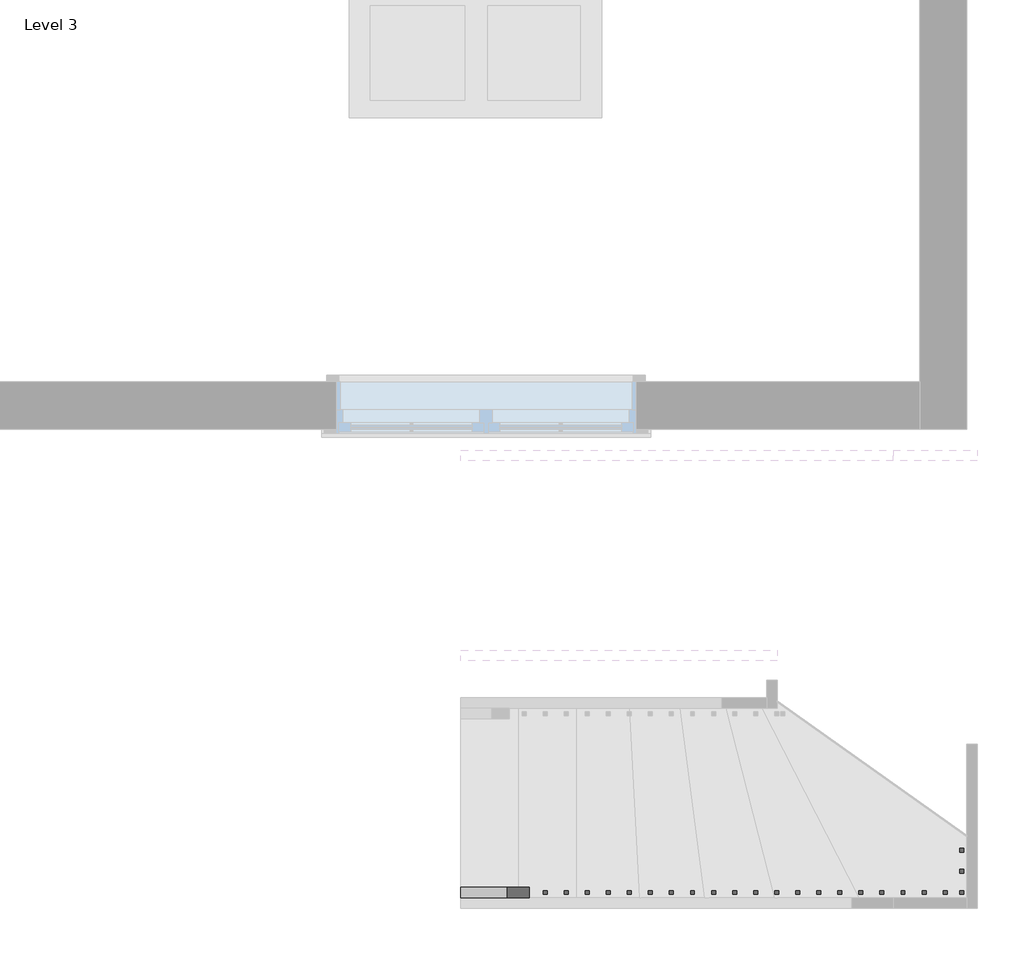
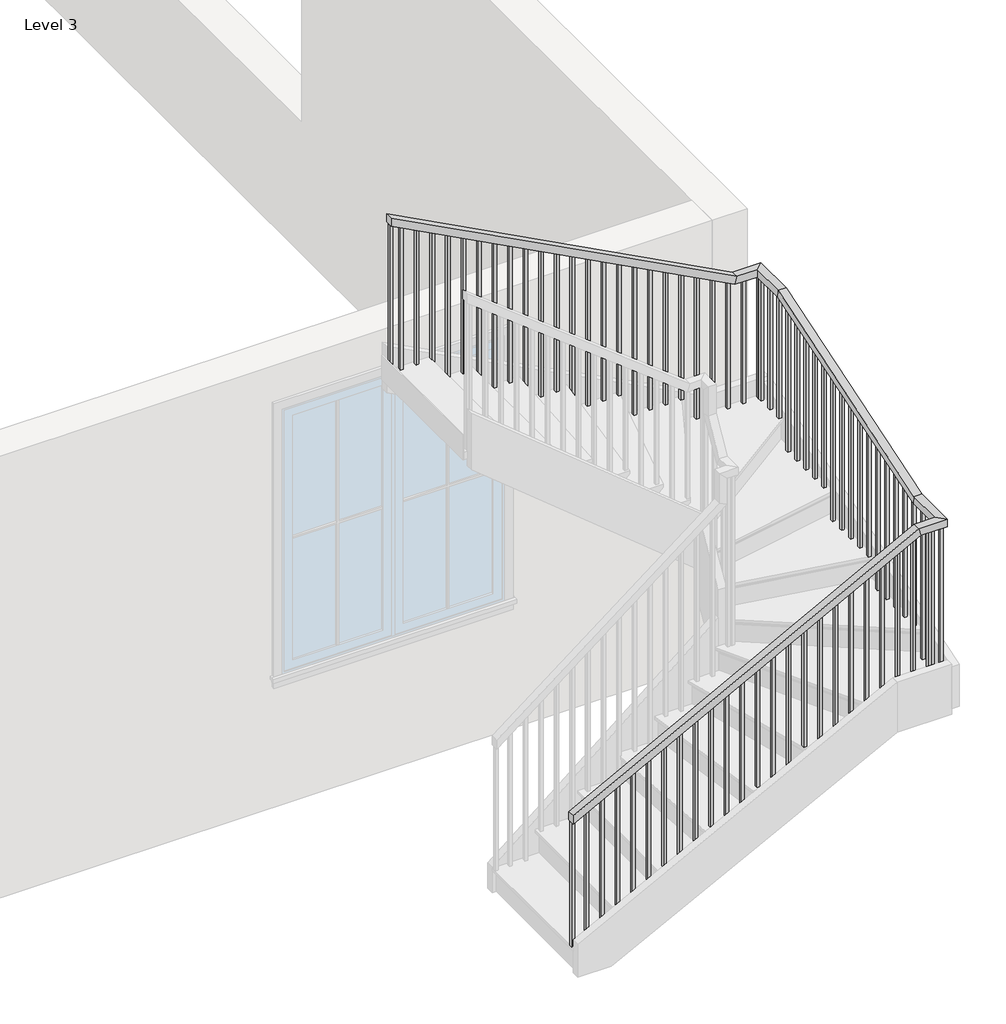
# One storey, part 2 of 3: 1 railing.
"""IFC4 building model written with IfcOpenShell, lengths in millimetres."""

from ifc_helpers import new_model, si_unit, frame, origin, place, context, project, spatial, polyline, outline, extrude, faceted_brep, element, save

model = new_model("IFC4")

# Units and contexts
model_context = context("Model", 3, world=origin())
ifc_project = project(units=[si_unit("LENGTHUNIT", "METRE", prefix="MILLI")], contexts=[model_context])

# Site, building, storey
site = spatial("IfcSite", under=ifc_project)
building = spatial("IfcBuilding", under=site)
storey = spatial("IfcBuildingStorey", under=building, Name="Level 3", Elevation=3200.4)

# Railing
placement = place(None, origin())
element("IfcRailing", 1, ObjectType="Handrail - Rectangular", at=placement, inside=storey, context=model_context, shape_type="SolidModel", body=[
    faceted_brep([(531.7538115, -7514.4090409, 4284.1333333), (531.7538115, -7514.4090409, 4226.6742652), (531.7538115, -7565.2090409, 4226.6742652), (531.7538115, -7565.2090409, 4284.1333333), (2789.4788736, -7514.4090409, 5477.4239201), (2802.0779381, -7514.4090409, 5426.6239201), (2802.0779381, -7565.2090409, 5426.6239201), (2789.4788736, -7565.2090409, 5477.4239201), (2923.0855034, -7269.9465826, 5426.6239201), (2923.0855034, -7277.8971587, 5477.4239201), (2923.0855034, -5744.320923, 5969.5094132), (2923.0855034, -5736.3703469, 5918.7094132), (2973.8855034, -7269.9465826, 5426.6239201), (2973.8855034, -5736.3703469, 5918.7094132), (2973.8855034, -7277.8971587, 5477.4239201), (2973.8855034, -5744.320923, 5969.5094132), (531.7538115, -5507.8090409, 7162.8), (531.7538115, -5457.0090409, 7162.8), (531.7538115, -5457.0090409, 7105.3409318), (531.7538115, -5507.8090409, 7105.3409318), (2776.879809, -5507.8090409, 5918.7094132), (2789.4788736, -5507.8090409, 5969.5094132), (2776.879809, -5457.0090409, 5918.7094132), (2789.4788736, -5457.0090409, 5969.5094132), (2923.0855034, -7514.4090409, 5477.4239201), (2923.0855034, -7514.4090409, 5426.6239201), (2973.8855034, -7565.2090409, 5426.6239201), (2973.8855034, -7565.2090409, 5477.4239201), (2923.0855034, -5507.8090409, 5969.5094132), (2923.0855034, -5507.8090409, 5918.7094132), (2973.8855034, -5457.0090409, 5918.7094132), (2973.8855034, -5457.0090409, 5969.5094132)], [[[0, 1, 2, 3]], [[1, 0, 4, 5]], [[2, 1, 5, 6]], [[3, 2, 6, 7]], [[0, 3, 7, 4]], [[8, 9, 10, 11]], [[12, 8, 11, 13]], [[14, 12, 13, 15]], [[9, 14, 15, 10]], [[16, 17, 18, 19]], [[20, 21, 16, 19]], [[22, 20, 19, 18]], [[23, 22, 18, 17]], [[21, 23, 17, 16]], [[5, 4, 24, 25]], [[6, 5, 25, 26]], [[7, 6, 26, 27]], [[4, 7, 27, 24]], [[25, 24, 9, 8]], [[26, 25, 8, 12]], [[27, 26, 12, 14]], [[24, 27, 14, 9]], [[11, 10, 28, 29]], [[13, 11, 29, 30]], [[15, 13, 30, 31]], [[10, 15, 31, 28]], [[29, 28, 21, 20]], [[30, 29, 20, 22]], [[31, 30, 22, 23]], [[28, 31, 23, 21]]]),
    extrude(outline(polyline([(7058.0597858, 621.2105034), (7068.1284102, 602.1605034), (6079.0666667, 602.1605034), (6079.0666667, 621.2105034), (7058.0597858, 621.2105034)])), frame((0.0, -5491.9340409, 0.0), z_axis=(0.0, 1.0, 0.0), x_axis=(0.0, 0.0, 1.0)), (0.0, 0.0, 1.0), 19.05),
    extrude(outline(polyline([(7004.3604556, 722.8105034), (7014.42908, 703.7605034), (6079.0666667, 703.7605034), (6079.0666667, 722.8105034), (7004.3604556, 722.8105034)])), frame((0.0, -5491.9340409, 0.0), z_axis=(0.0, 1.0, 0.0), x_axis=(0.0, 0.0, 1.0)), (0.0, 0.0, 1.0), 19.05),
    extrude(outline(polyline([(6950.6611254, 824.4105034), (6960.7297498, 805.3605034), (5909.7333333, 805.3605034), (5909.7333333, 824.4105034), (6950.6611254, 824.4105034)])), frame((0.0, -5491.9340409, 0.0), z_axis=(0.0, 1.0, 0.0), x_axis=(0.0, 0.0, 1.0)), (0.0, 0.0, 1.0), 19.05),
    extrude(outline(polyline([(6896.9617952, 926.0105034), (6907.0304196, 906.9605034), (5909.7333333, 906.9605034), (5909.7333333, 926.0105034), (6896.9617952, 926.0105034)])), frame((0.0, -5491.9340409, 0.0), z_axis=(0.0, 1.0, 0.0), x_axis=(0.0, 0.0, 1.0)), (0.0, 0.0, 1.0), 19.05),
    extrude(outline(polyline([(6843.262465, 1027.6105034), (6853.3310894, 1008.5605034), (5909.7333333, 1008.5605034), (5909.7333333, 1027.6105034), (6843.262465, 1027.6105034)])), frame((0.0, -5491.9340409, 0.0), z_axis=(0.0, 1.0, 0.0), x_axis=(0.0, 0.0, 1.0)), (0.0, 0.0, 1.0), 19.05),
    extrude(outline(polyline([(6789.5631348, 1129.2105034), (6799.6317592, 1110.1605034), (5740.4, 1110.1605034), (5740.4, 1129.2105034), (6789.5631348, 1129.2105034)])), frame((0.0, -5491.9340409, 0.0), z_axis=(0.0, 1.0, 0.0), x_axis=(0.0, 0.0, 1.0)), (0.0, 0.0, 1.0), 19.05),
    extrude(outline(polyline([(6735.8638046, 1230.8105034), (6745.932429, 1211.7605034), (5740.4, 1211.7605034), (5740.4, 1230.8105034), (6735.8638046, 1230.8105034)])), frame((0.0, -5491.9340409, 0.0), z_axis=(0.0, 1.0, 0.0), x_axis=(0.0, 0.0, 1.0)), (0.0, 0.0, 1.0), 19.05),
    extrude(outline(polyline([(6682.1644744, 1332.4105034), (6692.2330988, 1313.3605034), (5740.4, 1313.3605034), (5740.4, 1332.4105034), (6682.1644744, 1332.4105034)])), frame((0.0, -5491.9340409, 0.0), z_axis=(0.0, 1.0, 0.0), x_axis=(0.0, 0.0, 1.0)), (0.0, 0.0, 1.0), 19.05),
    extrude(outline(polyline([(6628.4651442, 1434.0105034), (6638.5337686, 1414.9605034), (5571.0666667, 1414.9605034), (5571.0666667, 1434.0105034), (6628.4651442, 1434.0105034)])), frame((0.0, -5491.9340409, 0.0), z_axis=(0.0, 1.0, 0.0), x_axis=(0.0, 0.0, 1.0)), (0.0, 0.0, 1.0), 19.05),
    extrude(outline(polyline([(6574.765814, 1535.6105034), (6584.8344384, 1516.5605034), (5571.0666667, 1516.5605034), (5571.0666667, 1535.6105034), (6574.765814, 1535.6105034)])), frame((0.0, -5491.9340409, 0.0), z_axis=(0.0, 1.0, 0.0), x_axis=(0.0, 0.0, 1.0)), (0.0, 0.0, 1.0), 19.05),
    extrude(outline(polyline([(6521.0664838, 1637.2105034), (6531.1351082, 1618.1605034), (5571.0666667, 1618.1605034), (5571.0666667, 1637.2105034), (6521.0664838, 1637.2105034)])), frame((0.0, -5491.9340409, 0.0), z_axis=(0.0, 1.0, 0.0), x_axis=(0.0, 0.0, 1.0)), (0.0, 0.0, 1.0), 19.05),
    extrude(outline(polyline([(6467.3671536, 1738.8105034), (6477.435778, 1719.7605034), (5401.7333333, 1719.7605034), (5401.7333333, 1738.8105034), (6467.3671536, 1738.8105034)])), frame((0.0, -5491.9340409, 0.0), z_axis=(0.0, 1.0, 0.0), x_axis=(0.0, 0.0, 1.0)), (0.0, 0.0, 1.0), 19.05),
    extrude(outline(polyline([(6413.6678234, 1840.4105034), (6423.7364478, 1821.3605034), (5401.7333333, 1821.3605034), (5401.7333333, 1840.4105034), (6413.6678234, 1840.4105034)])), frame((0.0, -5491.9340409, 0.0), z_axis=(0.0, 1.0, 0.0), x_axis=(0.0, 0.0, 1.0)), (0.0, 0.0, 1.0), 19.05),
    extrude(outline(polyline([(6359.9684932, 1942.0105034), (6370.0371176, 1922.9605034), (5401.7333333, 1922.9605034), (5401.7333333, 1942.0105034), (6359.9684932, 1942.0105034)])), frame((0.0, -5491.9340409, 0.0), z_axis=(0.0, 1.0, 0.0), x_axis=(0.0, 0.0, 1.0)), (0.0, 0.0, 1.0), 19.05),
    extrude(outline(polyline([(6306.269163, 2043.6105034), (6316.3377874, 2024.5605034), (5401.7333333, 2024.5605034), (5401.7333333, 2043.6105034), (6306.269163, 2043.6105034)])), frame((0.0, -5491.9340409, 0.0), z_axis=(0.0, 1.0, 0.0), x_axis=(0.0, 0.0, 1.0)), (0.0, 0.0, 1.0), 19.05),
    extrude(outline(polyline([(6252.5698328, 2145.2105034), (6262.6384572, 2126.1605034), (5232.4, 2126.1605034), (5232.4, 2145.2105034), (6252.5698328, 2145.2105034)])), frame((0.0, -5491.9340409, 0.0), z_axis=(0.0, 1.0, 0.0), x_axis=(0.0, 0.0, 1.0)), (0.0, 0.0, 1.0), 19.05),
    extrude(outline(polyline([(6198.8705026, 2246.8105034), (6208.939127, 2227.7605034), (5232.4, 2227.7605034), (5232.4, 2246.8105034), (6198.8705026, 2246.8105034)])), frame((0.0, -5491.9340409, 0.0), z_axis=(0.0, 1.0, 0.0), x_axis=(0.0, 0.0, 1.0)), (0.0, 0.0, 1.0), 19.05),
    extrude(outline(polyline([(6145.1711724, 2348.4105034), (6155.2397968, 2329.3605034), (5232.4, 2329.3605034), (5232.4, 2348.4105034), (6145.1711724, 2348.4105034)])), frame((0.0, -5491.9340409, 0.0), z_axis=(0.0, 1.0, 0.0), x_axis=(0.0, 0.0, 1.0)), (0.0, 0.0, 1.0), 19.05),
    extrude(outline(polyline([(6091.4718422, 2450.0105034), (6101.5404666, 2430.9605034), (5232.4, 2430.9605034), (5232.4, 2450.0105034), (6091.4718422, 2450.0105034)])), frame((0.0, -5491.9340409, 0.0), z_axis=(0.0, 1.0, 0.0), x_axis=(0.0, 0.0, 1.0)), (0.0, 0.0, 1.0), 19.05),
    extrude(outline(polyline([(6037.772512, 2551.6105034), (6047.8411364, 2532.5605034), (5063.0666667, 2532.5605034), (5063.0666667, 2551.6105034), (6037.772512, 2551.6105034)])), frame((0.0, -5491.9340409, 0.0), z_axis=(0.0, 1.0, 0.0), x_axis=(0.0, 0.0, 1.0)), (0.0, 0.0, 1.0), 19.05),
    extrude(outline(polyline([(5984.0731818, 2653.2105034), (5994.1418062, 2634.1605034), (5063.0666667, 2634.1605034), (5063.0666667, 2653.2105034), (5984.0731818, 2653.2105034)])), frame((0.0, -5491.9340409, 0.0), z_axis=(0.0, 1.0, 0.0), x_axis=(0.0, 0.0, 1.0)), (0.0, 0.0, 1.0), 19.05),
    extrude(outline(polyline([(5930.3738516, 2754.8105034), (5940.442476, 2735.7605034), (5063.0666667, 2735.7605034), (5063.0666667, 2754.8105034), (5930.3738516, 2754.8105034)])), frame((0.0, -5491.9340409, 0.0), z_axis=(0.0, 1.0, 0.0), x_axis=(0.0, 0.0, 1.0)), (0.0, 0.0, 1.0), 19.05),
    extrude(outline(polyline([(2856.4105034, -5472.8840409), (2856.4105034, -5491.9340409), (2837.3605034, -5491.9340409), (2837.3605034, -5472.8840409), (2856.4105034, -5472.8840409)])), frame((0.0, 0.0, 5063.0666667), z_axis=(0.0, 0.0, 1.0), x_axis=(1.0, 0.0, 0.0)), (0.0, 0.0, 1.0), 855.6427466),
    extrude(outline(polyline([(2958.0105034, -5517.3340409), (2938.9605034, -5517.3340409), (2938.9605034, -5498.2840409), (2958.0105034, -5498.2840409), (2958.0105034, -5517.3340409)])), frame((0.0, 0.0, 5063.0666667), z_axis=(0.0, 0.0, 1.0), x_axis=(1.0, 0.0, 0.0)), (0.0, 0.0, 1.0), 855.6427466),
    extrude(outline(polyline([(2958.0105034, -5618.9340409), (2938.9605034, -5618.9340409), (2938.9605034, -5599.8840409), (2958.0105034, -5599.8840409), (2958.0105034, -5618.9340409)])), frame((0.0, 0.0, 5063.0666667), z_axis=(0.0, 0.0, 1.0), x_axis=(1.0, 0.0, 0.0)), (0.0, 0.0, 1.0), 855.6427466),
    extrude(outline(polyline([(2958.0105034, -5720.5340409), (2938.9605034, -5720.5340409), (2938.9605034, -5701.4840409), (2958.0105034, -5701.4840409), (2958.0105034, -5720.5340409)])), frame((0.0, 0.0, 5063.0666667), z_axis=(0.0, 0.0, 1.0), x_axis=(1.0, 0.0, 0.0)), (0.0, 0.0, 1.0), 855.6427466),
    extrude(outline(polyline([(-5822.1340409, 5891.1900316), (-5803.0840409, 5897.3026907), (-5803.0840409, 4893.7333333), (-5822.1340409, 4893.7333333), (-5822.1340409, 5891.1900316)])), frame((2938.9605034, 0.0, 0.0), z_axis=(1.0, 0.0, 0.0), x_axis=(0.0, 1.0, 0.0)), (0.0, 0.0, 1.0), 19.05),
    extrude(outline(polyline([(-5923.7340409, 5858.5891834), (-5904.6840409, 5864.7018425), (-5904.6840409, 4893.7333333), (-5923.7340409, 4893.7333333), (-5923.7340409, 5858.5891834)])), frame((2938.9605034, 0.0, 0.0), z_axis=(1.0, 0.0, 0.0), x_axis=(0.0, 1.0, 0.0)), (0.0, 0.0, 1.0), 19.05),
    extrude(outline(polyline([(-6025.3340409, 5825.9883352), (-6006.2840409, 5832.1009942), (-6006.2840409, 4893.7333333), (-6025.3340409, 4893.7333333), (-6025.3340409, 5825.9883352)])), frame((2938.9605034, 0.0, 0.0), z_axis=(1.0, 0.0, 0.0), x_axis=(0.0, 1.0, 0.0)), (0.0, 0.0, 1.0), 19.05),
    extrude(outline(polyline([(-6126.9340409, 5793.387487), (-6107.8840409, 5799.500146), (-6107.8840409, 4893.7333333), (-6126.9340409, 4893.7333333), (-6126.9340409, 5793.387487)])), frame((2938.9605034, 0.0, 0.0), z_axis=(1.0, 0.0, 0.0), x_axis=(0.0, 1.0, 0.0)), (0.0, 0.0, 1.0), 19.05),
    extrude(outline(polyline([(-6228.5340409, 5760.7866387), (-6209.4840409, 5766.8992978), (-6209.4840409, 4893.7333333), (-6228.5340409, 4893.7333333), (-6228.5340409, 5760.7866387)])), frame((2938.9605034, 0.0, 0.0), z_axis=(1.0, 0.0, 0.0), x_axis=(0.0, 1.0, 0.0)), (0.0, 0.0, 1.0), 19.05),
    extrude(outline(polyline([(-6330.1340409, 5728.1857905), (-6311.0840409, 5734.2984495), (-6311.0840409, 4724.4), (-6330.1340409, 4724.4), (-6330.1340409, 5728.1857905)])), frame((2938.9605034, 0.0, 0.0), z_axis=(1.0, 0.0, 0.0), x_axis=(0.0, 1.0, 0.0)), (0.0, 0.0, 1.0), 19.05),
    extrude(outline(polyline([(-6431.7340409, 5695.5849423), (-6412.6840409, 5701.6976013), (-6412.6840409, 4724.4), (-6431.7340409, 4724.4), (-6431.7340409, 5695.5849423)])), frame((2938.9605034, 0.0, 0.0), z_axis=(1.0, 0.0, 0.0), x_axis=(0.0, 1.0, 0.0)), (0.0, 0.0, 1.0), 19.05),
    extrude(outline(polyline([(-6533.3340409, 5662.984094), (-6514.2840409, 5669.0967531), (-6514.2840409, 4724.4), (-6533.3340409, 4724.4), (-6533.3340409, 5662.984094)])), frame((2938.9605034, 0.0, 0.0), z_axis=(1.0, 0.0, 0.0), x_axis=(0.0, 1.0, 0.0)), (0.0, 0.0, 1.0), 19.05),
    extrude(outline(polyline([(-6634.9340409, 5630.3832458), (-6615.8840409, 5636.4959049), (-6615.8840409, 4724.4), (-6634.9340409, 4724.4), (-6634.9340409, 5630.3832458)])), frame((2938.9605034, 0.0, 0.0), z_axis=(1.0, 0.0, 0.0), x_axis=(0.0, 1.0, 0.0)), (0.0, 0.0, 1.0), 19.05),
    extrude(outline(polyline([(-6736.5340409, 5597.7823976), (-6717.4840409, 5603.8950566), (-6717.4840409, 4724.4), (-6736.5340409, 4724.4), (-6736.5340409, 5597.7823976)])), frame((2938.9605034, 0.0, 0.0), z_axis=(1.0, 0.0, 0.0), x_axis=(0.0, 1.0, 0.0)), (0.0, 0.0, 1.0), 19.05),
    extrude(outline(polyline([(-6838.1340409, 5565.1815494), (-6819.0840409, 5571.2942084), (-6819.0840409, 4555.0666667), (-6838.1340409, 4555.0666667), (-6838.1340409, 5565.1815494)])), frame((2938.9605034, 0.0, 0.0), z_axis=(1.0, 0.0, 0.0), x_axis=(0.0, 1.0, 0.0)), (0.0, 0.0, 1.0), 19.05),
    extrude(outline(polyline([(-6939.7340409, 5532.5807011), (-6920.6840409, 5538.6933602), (-6920.6840409, 4555.0666667), (-6939.7340409, 4555.0666667), (-6939.7340409, 5532.5807011)])), frame((2938.9605034, 0.0, 0.0), z_axis=(1.0, 0.0, 0.0), x_axis=(0.0, 1.0, 0.0)), (0.0, 0.0, 1.0), 19.05),
    extrude(outline(polyline([(-7041.3340409, 5499.9798529), (-7022.2840409, 5506.092512), (-7022.2840409, 4555.0666667), (-7041.3340409, 4555.0666667), (-7041.3340409, 5499.9798529)])), frame((2938.9605034, 0.0, 0.0), z_axis=(1.0, 0.0, 0.0), x_axis=(0.0, 1.0, 0.0)), (0.0, 0.0, 1.0), 19.05),
    extrude(outline(polyline([(-7142.9340409, 5467.3790047), (-7123.8840409, 5473.4916637), (-7123.8840409, 4555.0666667), (-7142.9340409, 4555.0666667), (-7142.9340409, 5467.3790047)])), frame((2938.9605034, 0.0, 0.0), z_axis=(1.0, 0.0, 0.0), x_axis=(0.0, 1.0, 0.0)), (0.0, 0.0, 1.0), 19.05),
    extrude(outline(polyline([(-7244.5340409, 5434.7781565), (-7225.4840409, 5440.8908155), (-7225.4840409, 4555.0666667), (-7244.5340409, 4555.0666667), (-7244.5340409, 5434.7781565)])), frame((2938.9605034, 0.0, 0.0), z_axis=(1.0, 0.0, 0.0), x_axis=(0.0, 1.0, 0.0)), (0.0, 0.0, 1.0), 19.05),
    extrude(outline(polyline([(2958.0105034, -7346.1340409), (2938.9605034, -7346.1340409), (2938.9605034, -7327.0840409), (2958.0105034, -7327.0840409), (2958.0105034, -7346.1340409)])), frame((0.0, 0.0, 4385.7333333), z_axis=(0.0, 0.0, 1.0), x_axis=(1.0, 0.0, 0.0)), (0.0, 0.0, 1.0), 1040.8905868),
    extrude(outline(polyline([(2958.0105034, -7447.7340409), (2938.9605034, -7447.7340409), (2938.9605034, -7428.6840409), (2958.0105034, -7428.6840409), (2958.0105034, -7447.7340409)])), frame((0.0, 0.0, 4385.7333333), z_axis=(0.0, 0.0, 1.0), x_axis=(1.0, 0.0, 0.0)), (0.0, 0.0, 1.0), 1040.8905868),
    extrude(outline(polyline([(2859.0288115, -7549.3340409), (2859.0288115, -7530.2840409), (2878.0788115, -7530.2840409), (2878.0788115, -7549.3340409), (2859.0288115, -7549.3340409)])), frame((0.0, 0.0, 4385.7333333), z_axis=(0.0, 0.0, 1.0), x_axis=(1.0, 0.0, 0.0)), (0.0, 0.0, 1.0), 1040.8905868),
    extrude(outline(polyline([(5413.0938418, 2776.4788115), (5403.0252174, 2757.4288115), (4385.7333333, 2757.4288115), (4385.7333333, 2776.4788115), (5413.0938418, 2776.4788115)])), frame((0.0, -7549.3340409, 0.0), z_axis=(0.0, 1.0, 0.0), x_axis=(0.0, 0.0, 1.0)), (0.0, 0.0, 1.0), 19.05),
    extrude(outline(polyline([(5359.3945116, 2674.8788115), (5349.3258872, 2655.8288115), (4385.7333333, 2655.8288115), (4385.7333333, 2674.8788115), (5359.3945116, 2674.8788115)])), frame((0.0, -7549.3340409, 0.0), z_axis=(0.0, 1.0, 0.0), x_axis=(0.0, 0.0, 1.0)), (0.0, 0.0, 1.0), 19.05),
    extrude(outline(polyline([(5305.6951814, 2573.2788115), (5295.626557, 2554.2288115), (4385.7333333, 2554.2288115), (4385.7333333, 2573.2788115), (5305.6951814, 2573.2788115)])), frame((0.0, -7549.3340409, 0.0), z_axis=(0.0, 1.0, 0.0), x_axis=(0.0, 0.0, 1.0)), (0.0, 0.0, 1.0), 19.05),
    extrude(outline(polyline([(5251.9958512, 2471.6788115), (5241.9272268, 2452.6288115), (4385.7333333, 2452.6288115), (4385.7333333, 2471.6788115), (5251.9958512, 2471.6788115)])), frame((0.0, -7549.3340409, 0.0), z_axis=(0.0, 1.0, 0.0), x_axis=(0.0, 0.0, 1.0)), (0.0, 0.0, 1.0), 19.05),
    extrude(outline(polyline([(5198.296521, 2370.0788115), (5188.2278966, 2351.0288115), (4216.4, 2351.0288115), (4216.4, 2370.0788115), (5198.296521, 2370.0788115)])), frame((0.0, -7549.3340409, 0.0), z_axis=(0.0, 1.0, 0.0), x_axis=(0.0, 0.0, 1.0)), (0.0, 0.0, 1.0), 19.05),
    extrude(outline(polyline([(5144.5971908, 2268.4788115), (5134.5285664, 2249.4288115), (4216.4, 2249.4288115), (4216.4, 2268.4788115), (5144.5971908, 2268.4788115)])), frame((0.0, -7549.3340409, 0.0), z_axis=(0.0, 1.0, 0.0), x_axis=(0.0, 0.0, 1.0)), (0.0, 0.0, 1.0), 19.05),
    extrude(outline(polyline([(5090.8978606, 2166.8788115), (5080.8292362, 2147.8288115), (4216.4, 2147.8288115), (4216.4, 2166.8788115), (5090.8978606, 2166.8788115)])), frame((0.0, -7549.3340409, 0.0), z_axis=(0.0, 1.0, 0.0), x_axis=(0.0, 0.0, 1.0)), (0.0, 0.0, 1.0), 19.05),
    extrude(outline(polyline([(5037.1985304, 2065.2788115), (5027.129906, 2046.2288115), (4216.4, 2046.2288115), (4216.4, 2065.2788115), (5037.1985304, 2065.2788115)])), frame((0.0, -7549.3340409, 0.0), z_axis=(0.0, 1.0, 0.0), x_axis=(0.0, 0.0, 1.0)), (0.0, 0.0, 1.0), 19.05),
    extrude(outline(polyline([(4983.4992002, 1963.6788115), (4973.4305758, 1944.6288115), (4047.0666667, 1944.6288115), (4047.0666667, 1963.6788115), (4983.4992002, 1963.6788115)])), frame((0.0, -7549.3340409, 0.0), z_axis=(0.0, 1.0, 0.0), x_axis=(0.0, 0.0, 1.0)), (0.0, 0.0, 1.0), 19.05),
    extrude(outline(polyline([(4929.79987, 1862.0788115), (4919.7312456, 1843.0288115), (4047.0666667, 1843.0288115), (4047.0666667, 1862.0788115), (4929.79987, 1862.0788115)])), frame((0.0, -7549.3340409, 0.0), z_axis=(0.0, 1.0, 0.0), x_axis=(0.0, 0.0, 1.0)), (0.0, 0.0, 1.0), 19.05),
    extrude(outline(polyline([(4876.1005398, 1760.4788115), (4866.0319154, 1741.4288115), (4047.0666667, 1741.4288115), (4047.0666667, 1760.4788115), (4876.1005398, 1760.4788115)])), frame((0.0, -7549.3340409, 0.0), z_axis=(0.0, 1.0, 0.0), x_axis=(0.0, 0.0, 1.0)), (0.0, 0.0, 1.0), 19.05),
    extrude(outline(polyline([(4822.4012096, 1658.8788115), (4812.3325852, 1639.8288115), (3877.7333333, 1639.8288115), (3877.7333333, 1658.8788115), (4822.4012096, 1658.8788115)])), frame((0.0, -7549.3340409, 0.0), z_axis=(0.0, 1.0, 0.0), x_axis=(0.0, 0.0, 1.0)), (0.0, 0.0, 1.0), 19.05),
    extrude(outline(polyline([(4768.7018794, 1557.2788115), (4758.633255, 1538.2288115), (3877.7333333, 1538.2288115), (3877.7333333, 1557.2788115), (4768.7018794, 1557.2788115)])), frame((0.0, -7549.3340409, 0.0), z_axis=(0.0, 1.0, 0.0), x_axis=(0.0, 0.0, 1.0)), (0.0, 0.0, 1.0), 19.05),
    extrude(outline(polyline([(4715.0025492, 1455.6788115), (4704.9339248, 1436.6288115), (3877.7333333, 1436.6288115), (3877.7333333, 1455.6788115), (4715.0025492, 1455.6788115)])), frame((0.0, -7549.3340409, 0.0), z_axis=(0.0, 1.0, 0.0), x_axis=(0.0, 0.0, 1.0)), (0.0, 0.0, 1.0), 19.05),
    extrude(outline(polyline([(4661.303219, 1354.0788115), (4651.2345946, 1335.0288115), (3708.4, 1335.0288115), (3708.4, 1354.0788115), (4661.303219, 1354.0788115)])), frame((0.0, -7549.3340409, 0.0), z_axis=(0.0, 1.0, 0.0), x_axis=(0.0, 0.0, 1.0)), (0.0, 0.0, 1.0), 19.05),
    extrude(outline(polyline([(4607.6038888, 1252.4788115), (4597.5352644, 1233.4288115), (3708.4, 1233.4288115), (3708.4, 1252.4788115), (4607.6038888, 1252.4788115)])), frame((0.0, -7549.3340409, 0.0), z_axis=(0.0, 1.0, 0.0), x_axis=(0.0, 0.0, 1.0)), (0.0, 0.0, 1.0), 19.05),
    extrude(outline(polyline([(4553.9045586, 1150.8788115), (4543.8359342, 1131.8288115), (3708.4, 1131.8288115), (3708.4, 1150.8788115), (4553.9045586, 1150.8788115)])), frame((0.0, -7549.3340409, 0.0), z_axis=(0.0, 1.0, 0.0), x_axis=(0.0, 0.0, 1.0)), (0.0, 0.0, 1.0), 19.05),
    extrude(outline(polyline([(4500.2052284, 1049.2788115), (4490.136604, 1030.2288115), (3539.0666667, 1030.2288115), (3539.0666667, 1049.2788115), (4500.2052284, 1049.2788115)])), frame((0.0, -7549.3340409, 0.0), z_axis=(0.0, 1.0, 0.0), x_axis=(0.0, 0.0, 1.0)), (0.0, 0.0, 1.0), 19.05),
    extrude(outline(polyline([(4446.5058982, 947.6788115), (4436.4372738, 928.6288115), (3539.0666667, 928.6288115), (3539.0666667, 947.6788115), (4446.5058982, 947.6788115)])), frame((0.0, -7549.3340409, 0.0), z_axis=(0.0, 1.0, 0.0), x_axis=(0.0, 0.0, 1.0)), (0.0, 0.0, 1.0), 19.05),
    extrude(outline(polyline([(4392.806568, 846.0788115), (4382.7379436, 827.0288115), (3539.0666667, 827.0288115), (3539.0666667, 846.0788115), (4392.806568, 846.0788115)])), frame((0.0, -7549.3340409, 0.0), z_axis=(0.0, 1.0, 0.0), x_axis=(0.0, 0.0, 1.0)), (0.0, 0.0, 1.0), 19.05),
    extrude(outline(polyline([(4339.1072378, 744.4788115), (4329.0386134, 725.4288115), (3369.7333333, 725.4288115), (3369.7333333, 744.4788115), (4339.1072378, 744.4788115)])), frame((0.0, -7549.3340409, 0.0), z_axis=(0.0, 1.0, 0.0), x_axis=(0.0, 0.0, 1.0)), (0.0, 0.0, 1.0), 19.05),
    extrude(outline(polyline([(4285.4079076, 642.8788115), (4275.3392831, 623.8288115), (3369.7333333, 623.8288115), (3369.7333333, 642.8788115), (4285.4079076, 642.8788115)])), frame((0.0, -7549.3340409, 0.0), z_axis=(0.0, 1.0, 0.0), x_axis=(0.0, 0.0, 1.0)), (0.0, 0.0, 1.0), 19.05),
    extrude(outline(polyline([(2958.0105034, -5491.9340409), (2938.9605034, -5491.9340409), (2938.9605034, -5472.8840409), (2958.0105034, -5472.8840409), (2958.0105034, -5491.9340409)])), frame((0.0, 0.0, 5063.0666667), z_axis=(0.0, 0.0, 1.0), x_axis=(1.0, 0.0, 0.0)), (0.0, 0.0, 1.0), 855.6427466),
    extrude(outline(polyline([(2938.9605034, -7549.3340409), (2938.9605034, -7530.2840409), (2958.0105034, -7530.2840409), (2958.0105034, -7549.3340409), (2938.9605034, -7549.3340409)])), frame((0.0, 0.0, 4385.7333333), z_axis=(0.0, 0.0, 1.0), x_axis=(1.0, 0.0, 0.0)), (0.0, 0.0, 1.0), 1040.8905868),
    extrude(outline(polyline([(7095.2723074, 550.8038115), (7105.3409318, 531.7538115), (6079.0666667, 531.7538115), (6079.0666667, 550.8038115), (7095.2723074, 550.8038115)])), frame((0.0, -5491.9340409, 0.0), z_axis=(0.0, 1.0, 0.0), x_axis=(0.0, 0.0, 1.0)), (0.0, 0.0, 1.0), 19.05),
    extrude(outline(polyline([(4236.7428896, 550.8038115), (4226.6742652, 531.7538115), (3369.7333333, 531.7538115), (3369.7333333, 550.8038115), (4236.7428896, 550.8038115)])), frame((0.0, -7549.3340409, 0.0), z_axis=(0.0, 1.0, 0.0), x_axis=(0.0, 0.0, 1.0)), (0.0, 0.0, 1.0), 19.05),
])

save(model, "model.ifc")

# Revit data of these elements
# Type "Handrail - Rectangular"
#   Assembly Code = "C2010400"
#   built-in parameter 1008612 = 0.0416667 (stored number, unit not read)
#   built-in parameter 1008611 = 0.0416667 (stored number, unit not read)
#   built-in parameter 1008609 = 0.333333 (stored number, unit not read)
#   built-in parameter 1008604 = 0.166667 (stored number, unit not read)
#   built-in parameter 1008603 = 0.166667 (stored number, unit not read)
#   Railing Height = 3' - 0"
#   built-in parameter 1008630 = 2
#   built-in parameter 1008610 = 2
#   built-in parameter 1008618 = Baluster - Square : 3/4"
# Element 1 (IfcRailing, "Handrail - Rectangular")
#   Phase Created = New Construction
